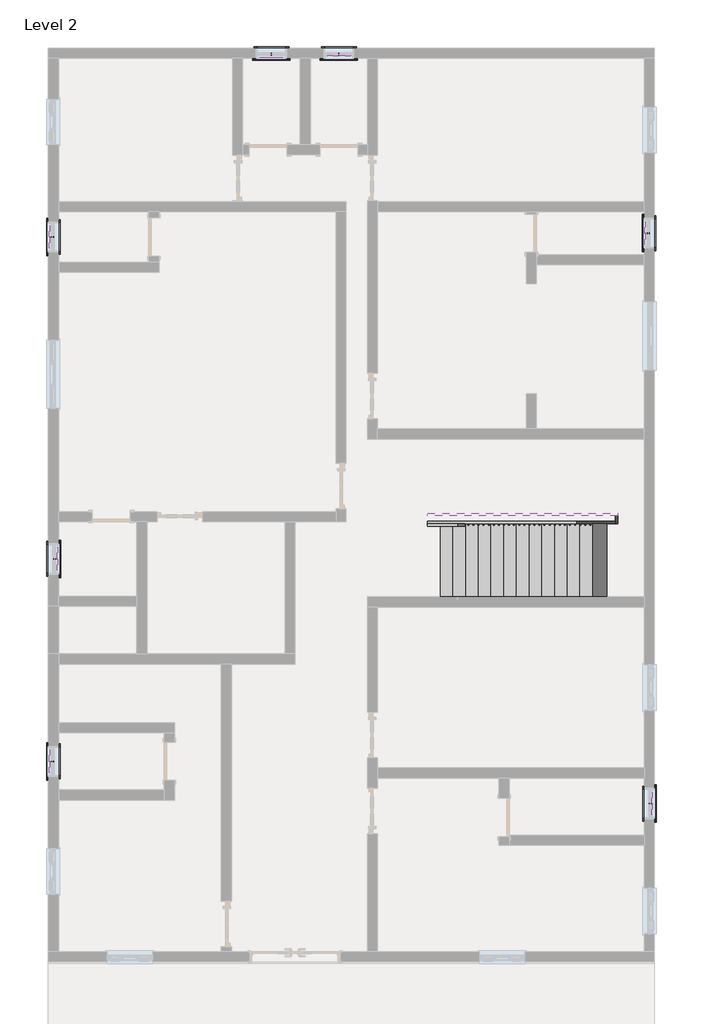
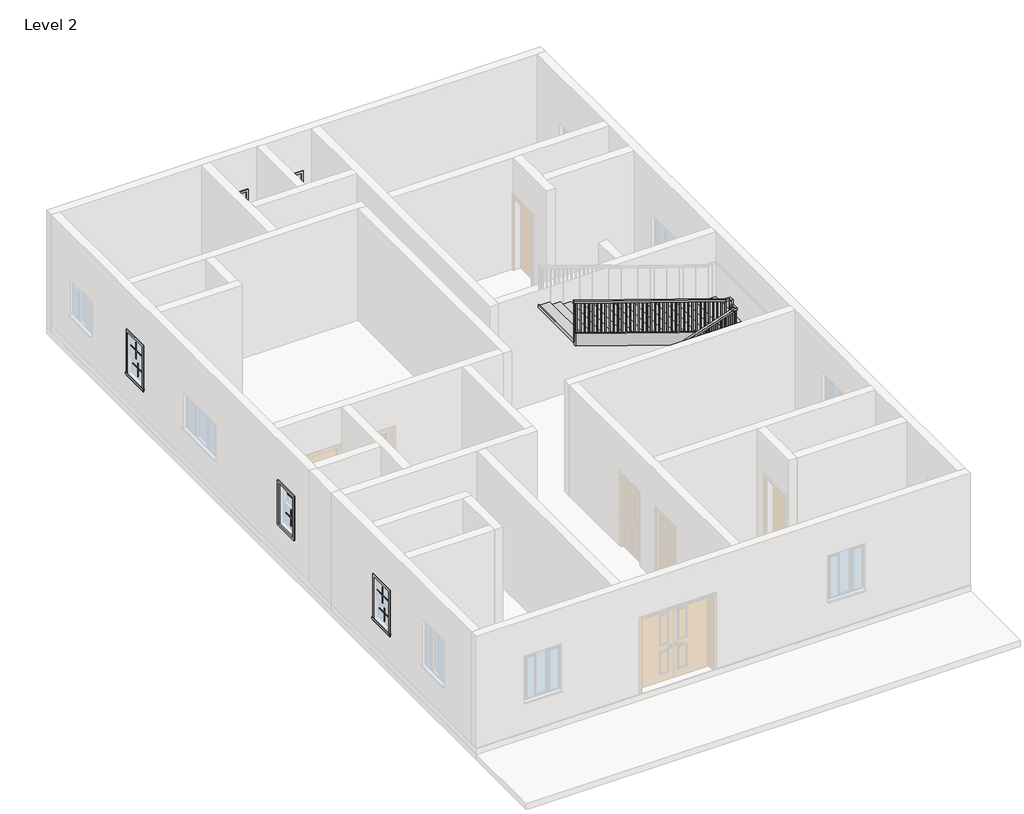
# One storey, part 3 of 3: 28 proxies, 6 members, 1 railing, 1 stair flight.
"""IFC4 building model written with IfcOpenShell, lengths in millimetres."""

from ifc_helpers import new_model, si_unit, frame, origin, place, context, project, spatial, polyline, outline, extrude, faceted_brep, transform, mapped, element, save
from components import muntin_pattern_2x2_muntin_pattern_2x2_eba6c5fb, trim_window_exterior_flat_with_sill_278e6a94, trim_window_interior_flat_picture_frame_e9fd5f45, stair_flight_4f1afc7f

model = new_model("IFC4")

# Units and contexts
model_context = context("Model", 3, world=origin())
ifc_project = project(units=[si_unit("LENGTHUNIT", "METRE", prefix="MILLI")], contexts=[model_context])

# Site, building, storey
site = spatial("IfcSite", under=ifc_project)
building = spatial("IfcBuilding", under=site)
storey = spatial("IfcBuildingStorey", under=building, Name="Level 2", Elevation=3048.0)

# Proxies
placement = place(None, origin())
muntin_pattern_2x2_muntin_pattern_2x2_shape = muntin_pattern_2x2_muntin_pattern_2x2_eba6c5fb(model_context)
element("IfcBuildingElementProxy", 1, Name="Muntin Pattern_2x2 : Muntin Pattern_2x2", ObjectType="Muntin Pattern_2x2 : Muntin Pattern_2x2", at=placement, inside=storey, context=model_context, shape_type="MappedRepresentation", body=[
    mapped(muntin_pattern_2x2_muntin_pattern_2x2_shape, transform((-6096.8589448, 5183.1303322, 4518.025), x_axis=(0.0, 1.0, 0.0), y_axis=(-1.0, 0.0, 0.0), z_axis=(0.0, 0.0, 1.0))),
])
element("IfcBuildingElementProxy", 2, Name="Muntin Pattern_2x2 : Muntin Pattern_2x2", ObjectType="Muntin Pattern_2x2 : Muntin Pattern_2x2", at=placement, inside=storey, context=model_context, shape_type="MappedRepresentation", body=[
    mapped(muntin_pattern_2x2_muntin_pattern_2x2_shape, transform((-6052.4089448, 5183.1303322, 4038.6), x_axis=(0.0, 1.0, 0.0), y_axis=(-1.0, 0.0, 0.0), z_axis=(0.0, 0.0, 1.0))),
])
element("IfcBuildingElementProxy", 3, Name="Muntin Pattern_2x2 : Muntin Pattern_2x2", ObjectType="Muntin Pattern_2x2 : Muntin Pattern_2x2", at=placement, inside=storey, context=model_context, shape_type="MappedRepresentation", body=[
    mapped(muntin_pattern_2x2_muntin_pattern_2x2_shape, transform((-1673.5309118, 8787.5224079, 4518.025), x_axis=(-1.0, 0.0, 0.0), y_axis=(0.0, -1.0, 0.0), z_axis=(0.0, 0.0, 1.0))),
])
element("IfcBuildingElementProxy", 4, Name="Muntin Pattern_2x2 : Muntin Pattern_2x2", ObjectType="Muntin Pattern_2x2 : Muntin Pattern_2x2", at=placement, inside=storey, context=model_context, shape_type="MappedRepresentation", body=[
    mapped(muntin_pattern_2x2_muntin_pattern_2x2_shape, transform((-1673.5309118, 8831.9724079, 4038.6), x_axis=(-1.0, 0.0, 0.0), y_axis=(0.0, -1.0, 0.0), z_axis=(0.0, 0.0, 1.0))),
])
element("IfcBuildingElementProxy", 5, Name="Muntin Pattern_2x2 : Muntin Pattern_2x2", ObjectType="Muntin Pattern_2x2 : Muntin Pattern_2x2", at=placement, inside=storey, context=model_context, shape_type="MappedRepresentation", body=[
    mapped(muntin_pattern_2x2_muntin_pattern_2x2_shape, transform((-324.5451949, 8787.5224079, 4518.025), x_axis=(-1.0, 0.0, 0.0), y_axis=(0.0, -1.0, 0.0), z_axis=(0.0, 0.0, 1.0))),
])
element("IfcBuildingElementProxy", 6, Name="Muntin Pattern_2x2 : Muntin Pattern_2x2", ObjectType="Muntin Pattern_2x2 : Muntin Pattern_2x2", at=placement, inside=storey, context=model_context, shape_type="MappedRepresentation", body=[
    mapped(muntin_pattern_2x2_muntin_pattern_2x2_shape, transform((-324.5451949, 8831.9724079, 4038.6), x_axis=(-1.0, 0.0, 0.0), y_axis=(0.0, -1.0, 0.0), z_axis=(0.0, 0.0, 1.0))),
])
element("IfcBuildingElementProxy", 7, Name="Muntin Pattern_2x2 : Muntin Pattern_2x2", ObjectType="Muntin Pattern_2x2 : Muntin Pattern_2x2", at=placement, inside=storey, context=model_context, shape_type="MappedRepresentation", body=[
    mapped(muntin_pattern_2x2_muntin_pattern_2x2_shape, transform((5813.4689795, 5259.3303322, 4518.025), x_axis=(0.0, 1.0, 0.0), y_axis=(-1.0, 0.0, 0.0), z_axis=(0.0, 0.0, 1.0))),
])
element("IfcBuildingElementProxy", 8, Name="Muntin Pattern_2x2 : Muntin Pattern_2x2", ObjectType="Muntin Pattern_2x2 : Muntin Pattern_2x2", at=placement, inside=storey, context=model_context, shape_type="MappedRepresentation", body=[
    mapped(muntin_pattern_2x2_muntin_pattern_2x2_shape, transform((5857.9189795, 5259.3303322, 4038.6), x_axis=(0.0, 1.0, 0.0), y_axis=(-1.0, 0.0, 0.0), z_axis=(0.0, 0.0, 1.0))),
])
element("IfcBuildingElementProxy", 9, Name="Muntin Pattern_2x2 : Muntin Pattern_2x2", ObjectType="Muntin Pattern_2x2 : Muntin Pattern_2x2", at=placement, inside=storey, context=model_context, shape_type="MappedRepresentation", body=[
    mapped(muntin_pattern_2x2_muntin_pattern_2x2_shape, transform((5946.8189795, -6133.2488489, 4518.025), x_axis=(0.0, -1.0, 0.0), y_axis=(1.0, 0.0, 0.0), z_axis=(0.0, 0.0, 1.0))),
])
element("IfcBuildingElementProxy", 10, Name="Muntin Pattern_2x2 : Muntin Pattern_2x2", ObjectType="Muntin Pattern_2x2 : Muntin Pattern_2x2", at=placement, inside=storey, context=model_context, shape_type="MappedRepresentation", body=[
    mapped(muntin_pattern_2x2_muntin_pattern_2x2_shape, transform((5902.3689795, -6133.2488489, 4038.6), x_axis=(0.0, -1.0, 0.0), y_axis=(1.0, 0.0, 0.0), z_axis=(0.0, 0.0, 1.0))),
])
element("IfcBuildingElementProxy", 11, Name="Muntin Pattern_2x2 : Muntin Pattern_2x2", ObjectType="Muntin Pattern_2x2 : Muntin Pattern_2x2", at=placement, inside=storey, context=model_context, shape_type="MappedRepresentation", body=[
    mapped(muntin_pattern_2x2_muntin_pattern_2x2_shape, transform((-6096.8589448, -5291.0659014, 4518.025), x_axis=(0.0, 1.0, 0.0), y_axis=(-1.0, 0.0, 0.0), z_axis=(0.0, 0.0, 1.0))),
])
element("IfcBuildingElementProxy", 12, Name="Muntin Pattern_2x2 : Muntin Pattern_2x2", ObjectType="Muntin Pattern_2x2 : Muntin Pattern_2x2", at=placement, inside=storey, context=model_context, shape_type="MappedRepresentation", body=[
    mapped(muntin_pattern_2x2_muntin_pattern_2x2_shape, transform((-6052.4089448, -5291.0659014, 4038.6), x_axis=(0.0, 1.0, 0.0), y_axis=(-1.0, 0.0, 0.0), z_axis=(0.0, 0.0, 1.0))),
])
element("IfcBuildingElementProxy", 13, Name="Muntin Pattern_2x2 : Muntin Pattern_2x2", ObjectType="Muntin Pattern_2x2 : Muntin Pattern_2x2", at=placement, inside=storey, context=model_context, shape_type="MappedRepresentation", body=[
    mapped(muntin_pattern_2x2_muntin_pattern_2x2_shape, transform((-5963.5089448, -1246.1159014, 4518.025), x_axis=(0.0, -1.0, 0.0), y_axis=(1.0, 0.0, 0.0), z_axis=(0.0, 0.0, 1.0))),
])
element("IfcBuildingElementProxy", 14, Name="Muntin Pattern_2x2 : Muntin Pattern_2x2", ObjectType="Muntin Pattern_2x2 : Muntin Pattern_2x2", at=placement, inside=storey, context=model_context, shape_type="MappedRepresentation", body=[
    mapped(muntin_pattern_2x2_muntin_pattern_2x2_shape, transform((-6007.9589448, -1246.1159014, 4038.6), x_axis=(0.0, -1.0, 0.0), y_axis=(1.0, 0.0, 0.0), z_axis=(0.0, 0.0, 1.0))),
])
trim_window_exterior_flat_with_sill_shape = trim_window_exterior_flat_with_sill_278e6a94(model_context)
element("IfcBuildingElementProxy", 15, Name="Trim-Window-Exterior-Flat : with Sill", ObjectType="Trim-Window-Exterior-Flat : with Sill", at=placement, inside=storey, context=model_context, shape_type="MappedRepresentation", body=[
    mapped(trim_window_exterior_flat_with_sill_shape, transform((-6131.7839448, 5183.1303322, 5029.2), x_axis=(0.0, -1.0, 0.0), y_axis=(0.0, 0.0, 1.0), z_axis=(-1.0, 0.0, 0.0))),
])
element("IfcBuildingElementProxy", 16, Name="Trim-Window-Exterior-Flat : with Sill", ObjectType="Trim-Window-Exterior-Flat : with Sill", at=placement, inside=storey, context=model_context, shape_type="MappedRepresentation", body=[
    mapped(trim_window_exterior_flat_with_sill_shape, transform((-1673.5309118, 8752.5974079, 5029.2), x_axis=(1.0, 0.0, 0.0), y_axis=(0.0, 0.0, 1.0), z_axis=(0.0, -1.0, 0.0))),
])
element("IfcBuildingElementProxy", 17, Name="Trim-Window-Exterior-Flat : with Sill", ObjectType="Trim-Window-Exterior-Flat : with Sill", at=placement, inside=storey, context=model_context, shape_type="MappedRepresentation", body=[
    mapped(trim_window_exterior_flat_with_sill_shape, transform((-324.5451949, 8752.5974079, 5029.2), x_axis=(1.0, 0.0, 0.0), y_axis=(0.0, 0.0, 1.0), z_axis=(0.0, -1.0, 0.0))),
])
element("IfcBuildingElementProxy", 18, Name="Trim-Window-Exterior-Flat : with Sill", ObjectType="Trim-Window-Exterior-Flat : with Sill", at=placement, inside=storey, context=model_context, shape_type="MappedRepresentation", body=[
    mapped(trim_window_exterior_flat_with_sill_shape, transform((5778.5439795, 5259.3303322, 5029.2), x_axis=(0.0, -1.0, 0.0), y_axis=(0.0, 0.0, 1.0), z_axis=(-1.0, 0.0, 0.0))),
])
element("IfcBuildingElementProxy", 19, Name="Trim-Window-Exterior-Flat : with Sill", ObjectType="Trim-Window-Exterior-Flat : with Sill", at=placement, inside=storey, context=model_context, shape_type="MappedRepresentation", body=[
    mapped(trim_window_exterior_flat_with_sill_shape, transform((5981.7439795, -6133.2488489, 5029.2), x_axis=(0.0, 1.0, 0.0), y_axis=(0.0, 0.0, 1.0), z_axis=(1.0, 0.0, 0.0))),
])
element("IfcBuildingElementProxy", 20, Name="Trim-Window-Exterior-Flat : with Sill", ObjectType="Trim-Window-Exterior-Flat : with Sill", at=placement, inside=storey, context=model_context, shape_type="MappedRepresentation", body=[
    mapped(trim_window_exterior_flat_with_sill_shape, transform((-6131.7839448, -5291.0659014, 5029.2), x_axis=(0.0, -1.0, 0.0), y_axis=(0.0, 0.0, 1.0), z_axis=(-1.0, 0.0, 0.0))),
])
element("IfcBuildingElementProxy", 21, Name="Trim-Window-Exterior-Flat : with Sill", ObjectType="Trim-Window-Exterior-Flat : with Sill", at=placement, inside=storey, context=model_context, shape_type="MappedRepresentation", body=[
    mapped(trim_window_exterior_flat_with_sill_shape, transform((-5928.5839448, -1246.1159014, 5029.2), x_axis=(0.0, 1.0, 0.0), y_axis=(0.0, 0.0, 1.0), z_axis=(1.0, 0.0, 0.0))),
])
trim_window_interior_flat_picture_frame_shape = trim_window_interior_flat_picture_frame_e9fd5f45(model_context)
element("IfcBuildingElementProxy", 22, Name="Trim-Window-Interior-Flat : Picture Frame", ObjectType="Trim-Window-Interior-Flat : Picture Frame", at=placement, inside=storey, context=model_context, shape_type="MappedRepresentation", body=[
    mapped(trim_window_interior_flat_picture_frame_shape, transform((-5928.5839448, 5183.1303322, 5029.2), x_axis=(0.0, 1.0, 0.0), y_axis=(0.0, 0.0, 1.0), z_axis=(1.0, 0.0, 0.0))),
])
element("IfcBuildingElementProxy", 23, Name="Trim-Window-Interior-Flat : Picture Frame", ObjectType="Trim-Window-Interior-Flat : Picture Frame", at=placement, inside=storey, context=model_context, shape_type="MappedRepresentation", body=[
    mapped(trim_window_interior_flat_picture_frame_shape, transform((-1673.5309118, 8955.7974079, 5029.2), x_axis=(-1.0, 0.0, 0.0), y_axis=(0.0, 0.0, 1.0), z_axis=(0.0, 1.0, 0.0))),
])
element("IfcBuildingElementProxy", 24, Name="Trim-Window-Interior-Flat : Picture Frame", ObjectType="Trim-Window-Interior-Flat : Picture Frame", at=placement, inside=storey, context=model_context, shape_type="MappedRepresentation", body=[
    mapped(trim_window_interior_flat_picture_frame_shape, transform((-324.5451949, 8955.7974079, 5029.2), x_axis=(-1.0, 0.0, 0.0), y_axis=(0.0, 0.0, 1.0), z_axis=(0.0, 1.0, 0.0))),
])
element("IfcBuildingElementProxy", 25, Name="Trim-Window-Interior-Flat : Picture Frame", ObjectType="Trim-Window-Interior-Flat : Picture Frame", at=placement, inside=storey, context=model_context, shape_type="MappedRepresentation", body=[
    mapped(trim_window_interior_flat_picture_frame_shape, transform((5981.7439795, 5259.3303322, 5029.2), x_axis=(0.0, 1.0, 0.0), y_axis=(0.0, 0.0, 1.0), z_axis=(1.0, 0.0, 0.0))),
])
element("IfcBuildingElementProxy", 26, Name="Trim-Window-Interior-Flat : Picture Frame", ObjectType="Trim-Window-Interior-Flat : Picture Frame", at=placement, inside=storey, context=model_context, shape_type="MappedRepresentation", body=[
    mapped(trim_window_interior_flat_picture_frame_shape, transform((5778.5439795, -6133.2488489, 5029.2), x_axis=(0.0, -1.0, 0.0), y_axis=(0.0, 0.0, 1.0), z_axis=(-1.0, 0.0, 0.0))),
])
element("IfcBuildingElementProxy", 27, Name="Trim-Window-Interior-Flat : Picture Frame", ObjectType="Trim-Window-Interior-Flat : Picture Frame", at=placement, inside=storey, context=model_context, shape_type="MappedRepresentation", body=[
    mapped(trim_window_interior_flat_picture_frame_shape, transform((-5928.5839448, -5291.0659014, 5029.2), x_axis=(0.0, 1.0, 0.0), y_axis=(0.0, 0.0, 1.0), z_axis=(1.0, 0.0, 0.0))),
])
element("IfcBuildingElementProxy", 28, Name="Trim-Window-Interior-Flat : Picture Frame", ObjectType="Trim-Window-Interior-Flat : Picture Frame", at=placement, inside=storey, context=model_context, shape_type="MappedRepresentation", body=[
    mapped(trim_window_interior_flat_picture_frame_shape, transform((-6131.7839448, -1246.1159014, 5029.2), x_axis=(0.0, -1.0, 0.0), y_axis=(0.0, 0.0, 1.0), z_axis=(-1.0, 0.0, 0.0))),
])

# Members
element("IfcMember", 29, ObjectType="Stringer - 2\" Width", at=placement, inside=storey, context=model_context, shape_type="SweptSolid", body=[
    extrude(outline(polyline([(3241.7751932, 1449.3932247), (3048.0, 1449.3932247), (3048.0, 1827.5890963), (4188.094539, 5195.8669505), (4495.8, 5195.8669505), (4495.8, 5154.2649181), (3241.7751932, 1449.3932247)])), frame((0.0, -541.2659014, 0.0), z_axis=(0.0, 1.0, 0.0), x_axis=(0.0, 0.0, 1.0)), (0.0, 0.0, 1.0), 50.8),
])
element("IfcMember", 30, ObjectType="Stringer - 2\" Width", at=placement, inside=storey, context=model_context, shape_type="SweptSolid", body=[
    extrude(outline(polyline([(5246.6669505, -541.2659014), (5195.8669505, -541.2659014), (5195.8669505, -388.7910016), (5246.6669505, -388.7910016), (5246.6669505, -541.2659014)])), frame((0.0, 0.0, 4191.0), z_axis=(0.0, 0.0, 1.0), x_axis=(1.0, 0.0, 0.0)), (0.0, 0.0, 1.0), 304.8),
])
element("IfcMember", 31, ObjectType="Stringer - 2\" Width", at=placement, inside=storey, context=model_context, shape_type="SweptSolid", body=[
    extrude(outline(polyline([(4291.0143208, 5246.6669505), (4612.8012358, 5246.6669505), (5898.1022784, 1449.3932247), (5576.3153634, 1449.3932247), (4291.0143208, 5246.6669505)])), frame((0.0, -388.7910016, 0.0), z_axis=(0.0, 1.0, 0.0), x_axis=(0.0, 0.0, 1.0)), (0.0, 0.0, 1.0), 50.8),
])
element("IfcMember", 32, ObjectType="Stringer - 2\" Width", at=placement, inside=storey, context=model_context, shape_type="SweptSolid", body=[
    extrude(outline(polyline([(3241.7751932, 1449.3932247), (3048.0, 1449.3932247), (3048.0, 1827.5890963), (4400.1142723, 5822.2548051), (4495.8, 5822.2548051), (4495.8, 5154.2649181), (3241.7751932, 1449.3932247)])), frame((0.0, -2116.0659014, 0.0), z_axis=(0.0, 1.0, 0.0), x_axis=(0.0, 0.0, 1.0)), (0.0, 0.0, 1.0), 50.8),
])
element("IfcMember", 33, ObjectType="Stringer - 2\" Width", at=placement, inside=storey, context=model_context, shape_type="SweptSolid", body=[
    extrude(outline(polyline([(5873.0548051, -2116.0659014), (5822.2548051, -2116.0659014), (5822.2548051, 1185.9340986), (5873.0548051, 1185.9340986), (5873.0548051, -2116.0659014)])), frame((0.0, 0.0, 4191.0), z_axis=(0.0, 0.0, 1.0), x_axis=(1.0, 0.0, 0.0)), (0.0, 0.0, 1.0), 304.8),
])
element("IfcMember", 34, ObjectType="Stringer - 2\" Width", at=placement, inside=storey, context=model_context, shape_type="SweptSolid", body=[
    extrude(outline(polyline([(4191.0, 5873.0548051), (4400.7815025, 5873.0548051), (5898.1022784, 1449.3932247), (5576.3153634, 1449.3932247), (4191.0, 5542.1477288), (4191.0, 5873.0548051)])), frame((0.0, 1185.9340986, 0.0), z_axis=(0.0, 1.0, 0.0), x_axis=(0.0, 0.0, 1.0)), (0.0, 0.0, 1.0), 50.8),
])

# Railing
element("IfcRailing", 35, ObjectType="Handrail - Rectangular", at=placement, inside=storey, context=model_context, shape_type="SolidModel", body=[
    faceted_brep([(1449.3932247, -541.2659014, 4048.125), (1449.3932247, -541.2659014, 3994.4913852), (1449.3932247, -592.0659014, 3994.4913852), (1449.3932247, -592.0659014, 4048.125), (5170.4669505, -541.2659014, 5308.1963098), (5221.2669505, -541.2659014, 5271.7651551), (5221.2669505, -592.0659014, 5271.7651551), (5170.4669505, -592.0659014, 5308.1963098), (5170.4669505, -541.2659014, 5334.0), (5221.2669505, -541.2659014, 5283.2), (5221.2669505, -592.0659014, 5283.2), (5170.4669505, -592.0659014, 5334.0), (5246.6669505, -541.2659014, 5334.0), (5246.6669505, -541.2659014, 5283.2), (5297.4669505, -592.0659014, 5283.2), (5297.4669505, -592.0659014, 5334.0), (5246.6669505, -465.0659014, 5334.0), (5246.6669505, -465.0659014, 5283.2), (5297.4669505, -465.0659014, 5283.2), (5297.4669505, -465.0659014, 5334.0), (5246.6669505, -414.1910016, 5334.0), (5246.6669505, -363.3910016, 5283.2), (5297.4669505, -363.3910016, 5283.2), (5297.4669505, -414.1910016, 5334.0), (5246.6669505, -414.1910016, 5445.5286902), (5246.6669505, -363.3910016, 5394.7286902), (5297.4669505, -363.3910016, 5394.7286902), (5297.4669505, -414.1910016, 5445.5286902), (5246.6669505, -337.9910016, 5445.5286902), (5246.6669505, -337.9910016, 5394.7286902), (5297.4669505, -287.1910016, 5394.7286902), (5297.4669505, -287.1910016, 5445.5286902), (5170.4669505, -337.9910016, 5445.5286902), (5162.099099, -337.9910016, 5394.7286902), (5162.099099, -287.1910016, 5394.7286902), (5170.4669505, -287.1910016, 5445.5286902), (1449.3932247, -337.9910016, 6705.6), (1449.3932247, -287.1910016, 6705.6), (1449.3932247, -287.1910016, 6651.9663852), (1449.3932247, -337.9910016, 6651.9663852)], [[[0, 1, 2, 3]], [[1, 0, 4, 5]], [[2, 1, 5, 6]], [[3, 2, 6, 7]], [[0, 3, 7, 4]], [[5, 4, 8, 9]], [[6, 5, 9, 10]], [[7, 6, 10, 11]], [[4, 7, 11, 8]], [[9, 8, 12, 13]], [[10, 9, 13, 14]], [[11, 10, 14, 15]], [[8, 11, 15, 12]], [[13, 12, 16, 17]], [[14, 13, 17, 18]], [[15, 14, 18, 19]], [[12, 15, 19, 16]], [[17, 16, 20, 21]], [[18, 17, 21, 22]], [[19, 18, 22, 23]], [[16, 19, 23, 20]], [[21, 20, 24, 25]], [[22, 21, 25, 26]], [[23, 22, 26, 27]], [[20, 23, 27, 24]], [[25, 24, 28, 29]], [[26, 25, 29, 30]], [[27, 26, 30, 31]], [[24, 27, 31, 28]], [[29, 28, 32, 33]], [[30, 29, 33, 34]], [[31, 30, 34, 35]], [[28, 31, 35, 32]], [[36, 37, 38, 39]], [[33, 32, 36, 39]], [[34, 33, 39, 38]], [[35, 34, 38, 37]], [[32, 35, 37, 36]]]),
    extrude(outline(polyline([(6633.6976686, 1503.3419505), (5705.475, 1503.3419505), (5705.475, 1522.3919505), (6627.246746, 1522.3919505), (6633.6976686, 1503.3419505)])), frame((0.0, -322.1160016, 0.0), z_axis=(0.0, 1.0, 0.0), x_axis=(0.0, 0.0, 1.0)), (0.0, 0.0, 1.0), 19.05),
    extrude(outline(polyline([(6599.2927482, 1604.9419505), (5705.475, 1604.9419505), (5705.475, 1623.9919505), (6592.8418257, 1623.9919505), (6599.2927482, 1604.9419505)])), frame((0.0, -322.1160016, 0.0), z_axis=(0.0, 1.0, 0.0), x_axis=(0.0, 0.0, 1.0)), (0.0, 0.0, 1.0), 19.05),
    extrude(outline(polyline([(6564.8878279, 1706.5419505), (5619.75, 1706.5419505), (5619.75, 1725.5919505), (6558.4369054, 1725.5919505), (6564.8878279, 1706.5419505)])), frame((0.0, -322.1160016, 0.0), z_axis=(0.0, 1.0, 0.0), x_axis=(0.0, 0.0, 1.0)), (0.0, 0.0, 1.0), 19.05),
    extrude(outline(polyline([(6530.4829076, 1808.1419505), (5619.75, 1808.1419505), (5619.75, 1827.1919505), (6524.031985, 1827.1919505), (6530.4829076, 1808.1419505)])), frame((0.0, -322.1160016, 0.0), z_axis=(0.0, 1.0, 0.0), x_axis=(0.0, 0.0, 1.0)), (0.0, 0.0, 1.0), 19.05),
    extrude(outline(polyline([(6496.0779873, 1909.7419505), (5619.75, 1909.7419505), (5619.75, 1928.7919505), (6489.6270647, 1928.7919505), (6496.0779873, 1909.7419505)])), frame((0.0, -322.1160016, 0.0), z_axis=(0.0, 1.0, 0.0), x_axis=(0.0, 0.0, 1.0)), (0.0, 0.0, 1.0), 19.05),
    extrude(outline(polyline([(6461.6730669, 2011.3419505), (5534.025, 2011.3419505), (5534.025, 2030.3919505), (6455.2221444, 2030.3919505), (6461.6730669, 2011.3419505)])), frame((0.0, -322.1160016, 0.0), z_axis=(0.0, 1.0, 0.0), x_axis=(0.0, 0.0, 1.0)), (0.0, 0.0, 1.0), 19.05),
    extrude(outline(polyline([(6427.2681466, 2112.9419505), (5534.025, 2112.9419505), (5534.025, 2131.9919505), (6420.817224, 2131.9919505), (6427.2681466, 2112.9419505)])), frame((0.0, -322.1160016, 0.0), z_axis=(0.0, 1.0, 0.0), x_axis=(0.0, 0.0, 1.0)), (0.0, 0.0, 1.0), 19.05),
    extrude(outline(polyline([(6392.8632263, 2214.5419505), (5448.3, 2214.5419505), (5448.3, 2233.5919505), (6386.4123037, 2233.5919505), (6392.8632263, 2214.5419505)])), frame((0.0, -322.1160016, 0.0), z_axis=(0.0, 1.0, 0.0), x_axis=(0.0, 0.0, 1.0)), (0.0, 0.0, 1.0), 19.05),
    extrude(outline(polyline([(6358.4583059, 2316.1419505), (5448.3, 2316.1419505), (5448.3, 2335.1919505), (6352.0073834, 2335.1919505), (6358.4583059, 2316.1419505)])), frame((0.0, -322.1160016, 0.0), z_axis=(0.0, 1.0, 0.0), x_axis=(0.0, 0.0, 1.0)), (0.0, 0.0, 1.0), 19.05),
    extrude(outline(polyline([(6324.0533856, 2417.7419505), (5448.3, 2417.7419505), (5448.3, 2436.7919505), (6317.6024631, 2436.7919505), (6324.0533856, 2417.7419505)])), frame((0.0, -322.1160016, 0.0), z_axis=(0.0, 1.0, 0.0), x_axis=(0.0, 0.0, 1.0)), (0.0, 0.0, 1.0), 19.05),
    extrude(outline(polyline([(6289.6484653, 2519.3419505), (5362.575, 2519.3419505), (5362.575, 2538.3919505), (6283.1975427, 2538.3919505), (6289.6484653, 2519.3419505)])), frame((0.0, -322.1160016, 0.0), z_axis=(0.0, 1.0, 0.0), x_axis=(0.0, 0.0, 1.0)), (0.0, 0.0, 1.0), 19.05),
    extrude(outline(polyline([(6255.243545, 2620.9419505), (5362.575, 2620.9419505), (5362.575, 2639.9919505), (6248.7926224, 2639.9919505), (6255.243545, 2620.9419505)])), frame((0.0, -322.1160016, 0.0), z_axis=(0.0, 1.0, 0.0), x_axis=(0.0, 0.0, 1.0)), (0.0, 0.0, 1.0), 19.05),
    extrude(outline(polyline([(6220.8386246, 2722.5419505), (5276.85, 2722.5419505), (5276.85, 2741.5919505), (6214.3877021, 2741.5919505), (6220.8386246, 2722.5419505)])), frame((0.0, -322.1160016, 0.0), z_axis=(0.0, 1.0, 0.0), x_axis=(0.0, 0.0, 1.0)), (0.0, 0.0, 1.0), 19.05),
    extrude(outline(polyline([(6186.4337043, 2824.1419505), (5276.85, 2824.1419505), (5276.85, 2843.1919505), (6179.9827817, 2843.1919505), (6186.4337043, 2824.1419505)])), frame((0.0, -322.1160016, 0.0), z_axis=(0.0, 1.0, 0.0), x_axis=(0.0, 0.0, 1.0)), (0.0, 0.0, 1.0), 19.05),
    extrude(outline(polyline([(6152.028784, 2925.7419505), (5276.85, 2925.7419505), (5276.85, 2944.7919505), (6145.5778614, 2944.7919505), (6152.028784, 2925.7419505)])), frame((0.0, -322.1160016, 0.0), z_axis=(0.0, 1.0, 0.0), x_axis=(0.0, 0.0, 1.0)), (0.0, 0.0, 1.0), 19.05),
    extrude(outline(polyline([(6117.6238636, 3027.3419505), (5191.125, 3027.3419505), (5191.125, 3046.3919505), (6111.1729411, 3046.3919505), (6117.6238636, 3027.3419505)])), frame((0.0, -322.1160016, 0.0), z_axis=(0.0, 1.0, 0.0), x_axis=(0.0, 0.0, 1.0)), (0.0, 0.0, 1.0), 19.05),
    extrude(outline(polyline([(6083.2189433, 3128.9419505), (5191.125, 3128.9419505), (5191.125, 3147.9919505), (6076.7680208, 3147.9919505), (6083.2189433, 3128.9419505)])), frame((0.0, -322.1160016, 0.0), z_axis=(0.0, 1.0, 0.0), x_axis=(0.0, 0.0, 1.0)), (0.0, 0.0, 1.0), 19.05),
    extrude(outline(polyline([(6048.814023, 3230.5419505), (5105.4, 3230.5419505), (5105.4, 3249.5919505), (6042.3631004, 3249.5919505), (6048.814023, 3230.5419505)])), frame((0.0, -322.1160016, 0.0), z_axis=(0.0, 1.0, 0.0), x_axis=(0.0, 0.0, 1.0)), (0.0, 0.0, 1.0), 19.05),
    extrude(outline(polyline([(6014.4091027, 3332.1419505), (5105.4, 3332.1419505), (5105.4, 3351.1919505), (6007.9581801, 3351.1919505), (6014.4091027, 3332.1419505)])), frame((0.0, -322.1160016, 0.0), z_axis=(0.0, 1.0, 0.0), x_axis=(0.0, 0.0, 1.0)), (0.0, 0.0, 1.0), 19.05),
    extrude(outline(polyline([(5980.0041823, 3433.7419505), (5105.4, 3433.7419505), (5105.4, 3452.7919505), (5973.5532598, 3452.7919505), (5980.0041823, 3433.7419505)])), frame((0.0, -322.1160016, 0.0), z_axis=(0.0, 1.0, 0.0), x_axis=(0.0, 0.0, 1.0)), (0.0, 0.0, 1.0), 19.05),
    extrude(outline(polyline([(5945.599262, 3535.3419505), (5019.675, 3535.3419505), (5019.675, 3554.3919505), (5939.1483394, 3554.3919505), (5945.599262, 3535.3419505)])), frame((0.0, -322.1160016, 0.0), z_axis=(0.0, 1.0, 0.0), x_axis=(0.0, 0.0, 1.0)), (0.0, 0.0, 1.0), 19.05),
    extrude(outline(polyline([(5911.1943417, 3636.9419505), (5019.675, 3636.9419505), (5019.675, 3655.9919505), (5904.7434191, 3655.9919505), (5911.1943417, 3636.9419505)])), frame((0.0, -322.1160016, 0.0), z_axis=(0.0, 1.0, 0.0), x_axis=(0.0, 0.0, 1.0)), (0.0, 0.0, 1.0), 19.05),
    extrude(outline(polyline([(5876.7894213, 3738.5419505), (4933.95, 3738.5419505), (4933.95, 3757.5919505), (5870.3384988, 3757.5919505), (5876.7894213, 3738.5419505)])), frame((0.0, -322.1160016, 0.0), z_axis=(0.0, 1.0, 0.0), x_axis=(0.0, 0.0, 1.0)), (0.0, 0.0, 1.0), 19.05),
    extrude(outline(polyline([(5842.384501, 3840.1419505), (4933.95, 3840.1419505), (4933.95, 3859.1919505), (5835.9335784, 3859.1919505), (5842.384501, 3840.1419505)])), frame((0.0, -322.1160016, 0.0), z_axis=(0.0, 1.0, 0.0), x_axis=(0.0, 0.0, 1.0)), (0.0, 0.0, 1.0), 19.05),
    extrude(outline(polyline([(5807.9795807, 3941.7419505), (4933.95, 3941.7419505), (4933.95, 3960.7919505), (5801.5286581, 3960.7919505), (5807.9795807, 3941.7419505)])), frame((0.0, -322.1160016, 0.0), z_axis=(0.0, 1.0, 0.0), x_axis=(0.0, 0.0, 1.0)), (0.0, 0.0, 1.0), 19.05),
    extrude(outline(polyline([(5773.5746604, 4043.3419505), (4848.225, 4043.3419505), (4848.225, 4062.3919505), (5767.1237378, 4062.3919505), (5773.5746604, 4043.3419505)])), frame((0.0, -322.1160016, 0.0), z_axis=(0.0, 1.0, 0.0), x_axis=(0.0, 0.0, 1.0)), (0.0, 0.0, 1.0), 19.05),
    extrude(outline(polyline([(5739.16974, 4144.9419505), (4848.225, 4144.9419505), (4848.225, 4163.9919505), (5732.7188175, 4163.9919505), (5739.16974, 4144.9419505)])), frame((0.0, -322.1160016, 0.0), z_axis=(0.0, 1.0, 0.0), x_axis=(0.0, 0.0, 1.0)), (0.0, 0.0, 1.0), 19.05),
    extrude(outline(polyline([(5704.7648197, 4246.5419505), (4762.5, 4246.5419505), (4762.5, 4265.5919505), (5698.3138971, 4265.5919505), (5704.7648197, 4246.5419505)])), frame((0.0, -322.1160016, 0.0), z_axis=(0.0, 1.0, 0.0), x_axis=(0.0, 0.0, 1.0)), (0.0, 0.0, 1.0), 19.05),
    extrude(outline(polyline([(5670.3598994, 4348.1419505), (4762.5, 4348.1419505), (4762.5, 4367.1919505), (5663.9089768, 4367.1919505), (5670.3598994, 4348.1419505)])), frame((0.0, -322.1160016, 0.0), z_axis=(0.0, 1.0, 0.0), x_axis=(0.0, 0.0, 1.0)), (0.0, 0.0, 1.0), 19.05),
    extrude(outline(polyline([(5635.954979, 4449.7419505), (4762.5, 4449.7419505), (4762.5, 4468.7919505), (5629.5040565, 4468.7919505), (5635.954979, 4449.7419505)])), frame((0.0, -322.1160016, 0.0), z_axis=(0.0, 1.0, 0.0), x_axis=(0.0, 0.0, 1.0)), (0.0, 0.0, 1.0), 19.05),
    extrude(outline(polyline([(5601.5500587, 4551.3419505), (4676.775, 4551.3419505), (4676.775, 4570.3919505), (5595.0991361, 4570.3919505), (5601.5500587, 4551.3419505)])), frame((0.0, -322.1160016, 0.0), z_axis=(0.0, 1.0, 0.0), x_axis=(0.0, 0.0, 1.0)), (0.0, 0.0, 1.0), 19.05),
    extrude(outline(polyline([(5567.1451384, 4652.9419505), (4676.775, 4652.9419505), (4676.775, 4671.9919505), (5560.6942158, 4671.9919505), (5567.1451384, 4652.9419505)])), frame((0.0, -322.1160016, 0.0), z_axis=(0.0, 1.0, 0.0), x_axis=(0.0, 0.0, 1.0)), (0.0, 0.0, 1.0), 19.05),
    extrude(outline(polyline([(5532.7402181, 4754.5419505), (4591.05, 4754.5419505), (4591.05, 4773.5919505), (5526.2892955, 4773.5919505), (5532.7402181, 4754.5419505)])), frame((0.0, -322.1160016, 0.0), z_axis=(0.0, 1.0, 0.0), x_axis=(0.0, 0.0, 1.0)), (0.0, 0.0, 1.0), 19.05),
    extrude(outline(polyline([(5498.3352977, 4856.1419505), (4591.05, 4856.1419505), (4591.05, 4875.1919505), (5491.8843752, 4875.1919505), (5498.3352977, 4856.1419505)])), frame((0.0, -322.1160016, 0.0), z_axis=(0.0, 1.0, 0.0), x_axis=(0.0, 0.0, 1.0)), (0.0, 0.0, 1.0), 19.05),
    extrude(outline(polyline([(5463.9303774, 4957.7419505), (4591.05, 4957.7419505), (4591.05, 4976.7919505), (5457.4794548, 4976.7919505), (5463.9303774, 4957.7419505)])), frame((0.0, -322.1160016, 0.0), z_axis=(0.0, 1.0, 0.0), x_axis=(0.0, 0.0, 1.0)), (0.0, 0.0, 1.0), 19.05),
    extrude(outline(polyline([(5429.5254571, 5059.3419505), (4505.325, 5059.3419505), (4505.325, 5078.3919505), (5423.0745345, 5078.3919505), (5429.5254571, 5059.3419505)])), frame((0.0, -322.1160016, 0.0), z_axis=(0.0, 1.0, 0.0), x_axis=(0.0, 0.0, 1.0)), (0.0, 0.0, 1.0), 19.05),
    extrude(outline(polyline([(5395.1205367, 5160.9419505), (4505.325, 5160.9419505), (4505.325, 5179.9919505), (5388.6696142, 5179.9919505), (5395.1205367, 5160.9419505)])), frame((0.0, -322.1160016, 0.0), z_axis=(0.0, 1.0, 0.0), x_axis=(0.0, 0.0, 1.0)), (0.0, 0.0, 1.0), 19.05),
    extrude(outline(polyline([(5262.5419505, -372.9909014), (5262.5419505, -353.9409014), (5281.5919505, -353.9409014), (5281.5919505, -372.9909014), (5262.5419505, -372.9909014)])), frame((0.0, 0.0, 4419.6), z_axis=(0.0, 0.0, 1.0), x_axis=(1.0, 0.0, 0.0)), (0.0, 0.0, 1.0), 975.1286902),
    extrude(outline(polyline([(5262.5419505, -474.5909014), (5262.5419505, -455.5409014), (5281.5919505, -455.5409014), (5281.5919505, -474.5909014), (5262.5419505, -474.5909014)])), frame((0.0, 0.0, 4419.6), z_axis=(0.0, 0.0, 1.0), x_axis=(1.0, 0.0, 0.0)), (0.0, 0.0, 1.0), 863.6),
    extrude(outline(polyline([(5199.0682247, -557.1409014), (5218.1182247, -557.1409014), (5218.1182247, -576.1909014), (5199.0682247, -576.1909014), (5199.0682247, -557.1409014)])), frame((0.0, 0.0, 4333.875), z_axis=(0.0, 0.0, 1.0), x_axis=(1.0, 0.0, 0.0)), (0.0, 0.0, 1.0), 949.325),
    extrude(outline(polyline([(5229.8430558, 5097.4682247), (4333.875, 5097.4682247), (4333.875, 5116.5182247), (5236.2939783, 5116.5182247), (5229.8430558, 5097.4682247)])), frame((0.0, -576.1909014, 0.0), z_axis=(0.0, 1.0, 0.0), x_axis=(0.0, 0.0, 1.0)), (0.0, 0.0, 1.0), 19.05),
    extrude(outline(polyline([(5195.4381354, 4995.8682247), (4333.875, 4995.8682247), (4333.875, 5014.9182247), (5201.889058, 5014.9182247), (5195.4381354, 4995.8682247)])), frame((0.0, -576.1909014, 0.0), z_axis=(0.0, 1.0, 0.0), x_axis=(0.0, 0.0, 1.0)), (0.0, 0.0, 1.0), 19.05),
    extrude(outline(polyline([(5161.0332151, 4894.2682247), (4248.15, 4894.2682247), (4248.15, 4913.3182247), (5167.4841377, 4913.3182247), (5161.0332151, 4894.2682247)])), frame((0.0, -576.1909014, 0.0), z_axis=(0.0, 1.0, 0.0), x_axis=(0.0, 0.0, 1.0)), (0.0, 0.0, 1.0), 19.05),
    extrude(outline(polyline([(5126.6282948, 4792.6682247), (4248.15, 4792.6682247), (4248.15, 4811.7182247), (5133.0792173, 4811.7182247), (5126.6282948, 4792.6682247)])), frame((0.0, -576.1909014, 0.0), z_axis=(0.0, 1.0, 0.0), x_axis=(0.0, 0.0, 1.0)), (0.0, 0.0, 1.0), 19.05),
    extrude(outline(polyline([(5092.2233745, 4691.0682247), (4162.425, 4691.0682247), (4162.425, 4710.1182247), (5098.674297, 4710.1182247), (5092.2233745, 4691.0682247)])), frame((0.0, -576.1909014, 0.0), z_axis=(0.0, 1.0, 0.0), x_axis=(0.0, 0.0, 1.0)), (0.0, 0.0, 1.0), 19.05),
    extrude(outline(polyline([(5057.8184541, 4589.4682247), (4162.425, 4589.4682247), (4162.425, 4608.5182247), (5064.2693767, 4608.5182247), (5057.8184541, 4589.4682247)])), frame((0.0, -576.1909014, 0.0), z_axis=(0.0, 1.0, 0.0), x_axis=(0.0, 0.0, 1.0)), (0.0, 0.0, 1.0), 19.05),
    extrude(outline(polyline([(5023.4135338, 4487.8682247), (4162.425, 4487.8682247), (4162.425, 4506.9182247), (5029.8644564, 4506.9182247), (5023.4135338, 4487.8682247)])), frame((0.0, -576.1909014, 0.0), z_axis=(0.0, 1.0, 0.0), x_axis=(0.0, 0.0, 1.0)), (0.0, 0.0, 1.0), 19.05),
    extrude(outline(polyline([(4989.0086135, 4386.2682247), (4076.7, 4386.2682247), (4076.7, 4405.3182247), (4995.459536, 4405.3182247), (4989.0086135, 4386.2682247)])), frame((0.0, -576.1909014, 0.0), z_axis=(0.0, 1.0, 0.0), x_axis=(0.0, 0.0, 1.0)), (0.0, 0.0, 1.0), 19.05),
    extrude(outline(polyline([(4954.6036931, 4284.6682247), (4076.7, 4284.6682247), (4076.7, 4303.7182247), (4961.0546157, 4303.7182247), (4954.6036931, 4284.6682247)])), frame((0.0, -576.1909014, 0.0), z_axis=(0.0, 1.0, 0.0), x_axis=(0.0, 0.0, 1.0)), (0.0, 0.0, 1.0), 19.05),
    extrude(outline(polyline([(4920.1987728, 4183.0682247), (3990.975, 4183.0682247), (3990.975, 4202.1182247), (4926.6496954, 4202.1182247), (4920.1987728, 4183.0682247)])), frame((0.0, -576.1909014, 0.0), z_axis=(0.0, 1.0, 0.0), x_axis=(0.0, 0.0, 1.0)), (0.0, 0.0, 1.0), 19.05),
    extrude(outline(polyline([(4885.7938525, 4081.4682247), (3990.975, 4081.4682247), (3990.975, 4100.5182247), (4892.244775, 4100.5182247), (4885.7938525, 4081.4682247)])), frame((0.0, -576.1909014, 0.0), z_axis=(0.0, 1.0, 0.0), x_axis=(0.0, 0.0, 1.0)), (0.0, 0.0, 1.0), 19.05),
    extrude(outline(polyline([(4851.3889321, 3979.8682247), (3990.975, 3979.8682247), (3990.975, 3998.9182247), (4857.8398547, 3998.9182247), (4851.3889321, 3979.8682247)])), frame((0.0, -576.1909014, 0.0), z_axis=(0.0, 1.0, 0.0), x_axis=(0.0, 0.0, 1.0)), (0.0, 0.0, 1.0), 19.05),
    extrude(outline(polyline([(4816.9840118, 3878.2682247), (3905.25, 3878.2682247), (3905.25, 3897.3182247), (4823.4349344, 3897.3182247), (4816.9840118, 3878.2682247)])), frame((0.0, -576.1909014, 0.0), z_axis=(0.0, 1.0, 0.0), x_axis=(0.0, 0.0, 1.0)), (0.0, 0.0, 1.0), 19.05),
    extrude(outline(polyline([(4782.5790915, 3776.6682247), (3905.25, 3776.6682247), (3905.25, 3795.7182247), (4789.0300141, 3795.7182247), (4782.5790915, 3776.6682247)])), frame((0.0, -576.1909014, 0.0), z_axis=(0.0, 1.0, 0.0), x_axis=(0.0, 0.0, 1.0)), (0.0, 0.0, 1.0), 19.05),
    extrude(outline(polyline([(4748.1741712, 3675.0682247), (3819.525, 3675.0682247), (3819.525, 3694.1182247), (4754.6250937, 3694.1182247), (4748.1741712, 3675.0682247)])), frame((0.0, -576.1909014, 0.0), z_axis=(0.0, 1.0, 0.0), x_axis=(0.0, 0.0, 1.0)), (0.0, 0.0, 1.0), 19.05),
    extrude(outline(polyline([(4713.7692508, 3573.4682247), (3819.525, 3573.4682247), (3819.525, 3592.5182247), (4720.2201734, 3592.5182247), (4713.7692508, 3573.4682247)])), frame((0.0, -576.1909014, 0.0), z_axis=(0.0, 1.0, 0.0), x_axis=(0.0, 0.0, 1.0)), (0.0, 0.0, 1.0), 19.05),
    extrude(outline(polyline([(4679.3643305, 3471.8682247), (3819.525, 3471.8682247), (3819.525, 3490.9182247), (4685.8152531, 3490.9182247), (4679.3643305, 3471.8682247)])), frame((0.0, -576.1909014, 0.0), z_axis=(0.0, 1.0, 0.0), x_axis=(0.0, 0.0, 1.0)), (0.0, 0.0, 1.0), 19.05),
    extrude(outline(polyline([(4644.9594102, 3370.2682247), (3733.8, 3370.2682247), (3733.8, 3389.3182247), (4651.4103327, 3389.3182247), (4644.9594102, 3370.2682247)])), frame((0.0, -576.1909014, 0.0), z_axis=(0.0, 1.0, 0.0), x_axis=(0.0, 0.0, 1.0)), (0.0, 0.0, 1.0), 19.05),
    extrude(outline(polyline([(4610.5544898, 3268.6682247), (3733.8, 3268.6682247), (3733.8, 3287.7182247), (4617.0054124, 3287.7182247), (4610.5544898, 3268.6682247)])), frame((0.0, -576.1909014, 0.0), z_axis=(0.0, 1.0, 0.0), x_axis=(0.0, 0.0, 1.0)), (0.0, 0.0, 1.0), 19.05),
    extrude(outline(polyline([(4576.1495695, 3167.0682247), (3648.075, 3167.0682247), (3648.075, 3186.1182247), (4582.6004921, 3186.1182247), (4576.1495695, 3167.0682247)])), frame((0.0, -576.1909014, 0.0), z_axis=(0.0, 1.0, 0.0), x_axis=(0.0, 0.0, 1.0)), (0.0, 0.0, 1.0), 19.05),
    extrude(outline(polyline([(4541.7446492, 3065.4682247), (3648.075, 3065.4682247), (3648.075, 3084.5182247), (4548.1955718, 3084.5182247), (4541.7446492, 3065.4682247)])), frame((0.0, -576.1909014, 0.0), z_axis=(0.0, 1.0, 0.0), x_axis=(0.0, 0.0, 1.0)), (0.0, 0.0, 1.0), 19.05),
    extrude(outline(polyline([(4507.3397289, 2963.8682247), (3648.075, 2963.8682247), (3648.075, 2982.9182247), (4513.7906514, 2982.9182247), (4507.3397289, 2963.8682247)])), frame((0.0, -576.1909014, 0.0), z_axis=(0.0, 1.0, 0.0), x_axis=(0.0, 0.0, 1.0)), (0.0, 0.0, 1.0), 19.05),
    extrude(outline(polyline([(4472.9348085, 2862.2682247), (3562.35, 2862.2682247), (3562.35, 2881.3182247), (4479.3857311, 2881.3182247), (4472.9348085, 2862.2682247)])), frame((0.0, -576.1909014, 0.0), z_axis=(0.0, 1.0, 0.0), x_axis=(0.0, 0.0, 1.0)), (0.0, 0.0, 1.0), 19.05),
    extrude(outline(polyline([(4438.5298882, 2760.6682247), (3562.35, 2760.6682247), (3562.35, 2779.7182247), (4444.9808108, 2779.7182247), (4438.5298882, 2760.6682247)])), frame((0.0, -576.1909014, 0.0), z_axis=(0.0, 1.0, 0.0), x_axis=(0.0, 0.0, 1.0)), (0.0, 0.0, 1.0), 19.05),
    extrude(outline(polyline([(4404.1249679, 2659.0682247), (3476.625, 2659.0682247), (3476.625, 2678.1182247), (4410.5758904, 2678.1182247), (4404.1249679, 2659.0682247)])), frame((0.0, -576.1909014, 0.0), z_axis=(0.0, 1.0, 0.0), x_axis=(0.0, 0.0, 1.0)), (0.0, 0.0, 1.0), 19.05),
    extrude(outline(polyline([(4369.7200475, 2557.4682247), (3476.625, 2557.4682247), (3476.625, 2576.5182247), (4376.1709701, 2576.5182247), (4369.7200475, 2557.4682247)])), frame((0.0, -576.1909014, 0.0), z_axis=(0.0, 1.0, 0.0), x_axis=(0.0, 0.0, 1.0)), (0.0, 0.0, 1.0), 19.05),
    extrude(outline(polyline([(4335.3151272, 2455.8682247), (3476.625, 2455.8682247), (3476.625, 2474.9182247), (4341.7660498, 2474.9182247), (4335.3151272, 2455.8682247)])), frame((0.0, -576.1909014, 0.0), z_axis=(0.0, 1.0, 0.0), x_axis=(0.0, 0.0, 1.0)), (0.0, 0.0, 1.0), 19.05),
    extrude(outline(polyline([(4300.9102069, 2354.2682247), (3390.9, 2354.2682247), (3390.9, 2373.3182247), (4307.3611294, 2373.3182247), (4300.9102069, 2354.2682247)])), frame((0.0, -576.1909014, 0.0), z_axis=(0.0, 1.0, 0.0), x_axis=(0.0, 0.0, 1.0)), (0.0, 0.0, 1.0), 19.05),
    extrude(outline(polyline([(4266.5052866, 2252.6682247), (3390.9, 2252.6682247), (3390.9, 2271.7182247), (4272.9562091, 2271.7182247), (4266.5052866, 2252.6682247)])), frame((0.0, -576.1909014, 0.0), z_axis=(0.0, 1.0, 0.0), x_axis=(0.0, 0.0, 1.0)), (0.0, 0.0, 1.0), 19.05),
    extrude(outline(polyline([(4232.1003662, 2151.0682247), (3305.175, 2151.0682247), (3305.175, 2170.1182247), (4238.5512888, 2170.1182247), (4232.1003662, 2151.0682247)])), frame((0.0, -576.1909014, 0.0), z_axis=(0.0, 1.0, 0.0), x_axis=(0.0, 0.0, 1.0)), (0.0, 0.0, 1.0), 19.05),
    extrude(outline(polyline([(4197.6954459, 2049.4682247), (3305.175, 2049.4682247), (3305.175, 2068.5182247), (4204.1463685, 2068.5182247), (4197.6954459, 2049.4682247)])), frame((0.0, -576.1909014, 0.0), z_axis=(0.0, 1.0, 0.0), x_axis=(0.0, 0.0, 1.0)), (0.0, 0.0, 1.0), 19.05),
    extrude(outline(polyline([(4163.2905256, 1947.8682247), (3305.175, 1947.8682247), (3305.175, 1966.9182247), (4169.7414481, 1966.9182247), (4163.2905256, 1947.8682247)])), frame((0.0, -576.1909014, 0.0), z_axis=(0.0, 1.0, 0.0), x_axis=(0.0, 0.0, 1.0)), (0.0, 0.0, 1.0), 19.05),
    extrude(outline(polyline([(4128.8856052, 1846.2682247), (3219.45, 1846.2682247), (3219.45, 1865.3182247), (4135.3365278, 1865.3182247), (4128.8856052, 1846.2682247)])), frame((0.0, -576.1909014, 0.0), z_axis=(0.0, 1.0, 0.0), x_axis=(0.0, 0.0, 1.0)), (0.0, 0.0, 1.0), 19.05),
    extrude(outline(polyline([(4094.4806849, 1744.6682247), (3219.45, 1744.6682247), (3219.45, 1763.7182247), (4100.9316075, 1763.7182247), (4094.4806849, 1744.6682247)])), frame((0.0, -576.1909014, 0.0), z_axis=(0.0, 1.0, 0.0), x_axis=(0.0, 0.0, 1.0)), (0.0, 0.0, 1.0), 19.05),
    extrude(outline(polyline([(4060.0757646, 1643.0682247), (3133.725, 1643.0682247), (3133.725, 1662.1182247), (4066.5266871, 1662.1182247), (4060.0757646, 1643.0682247)])), frame((0.0, -576.1909014, 0.0), z_axis=(0.0, 1.0, 0.0), x_axis=(0.0, 0.0, 1.0)), (0.0, 0.0, 1.0), 19.05),
    extrude(outline(polyline([(4025.6708443, 1541.4682247), (3133.725, 1541.4682247), (3133.725, 1560.5182247), (4032.1217668, 1560.5182247), (4025.6708443, 1541.4682247)])), frame((0.0, -576.1909014, 0.0), z_axis=(0.0, 1.0, 0.0), x_axis=(0.0, 0.0, 1.0)), (0.0, 0.0, 1.0), 19.05),
    extrude(outline(polyline([(5262.5419505, -322.1160016), (5262.5419505, -303.0660016), (5281.5919505, -303.0660016), (5281.5919505, -322.1160016), (5262.5419505, -322.1160016)])), frame((0.0, 0.0, 4419.6), z_axis=(0.0, 0.0, 1.0), x_axis=(1.0, 0.0, 0.0)), (0.0, 0.0, 1.0), 975.1286902),
    extrude(outline(polyline([(5262.5419505, -557.1409014), (5281.5919505, -557.1409014), (5281.5919505, -576.1909014), (5262.5419505, -576.1909014), (5262.5419505, -557.1409014)])), frame((0.0, 0.0, 4419.6), z_axis=(0.0, 0.0, 1.0), x_axis=(1.0, 0.0, 0.0)), (0.0, 0.0, 1.0), 863.6),
    extrude(outline(polyline([(6651.9663852, 1449.3932247), (5705.475, 1449.3932247), (5705.475, 1468.4432247), (6645.5154626, 1468.4432247), (6651.9663852, 1449.3932247)])), frame((0.0, -322.1160016, 0.0), z_axis=(0.0, 1.0, 0.0), x_axis=(0.0, 0.0, 1.0)), (0.0, 0.0, 1.0), 19.05),
    extrude(outline(polyline([(3994.4913852, 1449.3932247), (3133.725, 1449.3932247), (3133.725, 1468.4432247), (4000.9423078, 1468.4432247), (3994.4913852, 1449.3932247)])), frame((0.0, -576.1909014, 0.0), z_axis=(0.0, 1.0, 0.0), x_axis=(0.0, 0.0, 1.0)), (0.0, 0.0, 1.0), 19.05),
])

# Stair flight
stair_flight_shape = stair_flight_4f1afc7f(model_context)
element("IfcStairFlight", 36, ObjectType="2\" Tread 1\" Nosing 1/4\" Riser", at=placement, inside=storey, context=model_context, shape_type="MappedRepresentation", body=[
    mapped(stair_flight_shape, transform((0.0, 0.0, 0.0), x_axis=(1.0, 0.0, 0.0), y_axis=(0.0, 1.0, 0.0), z_axis=(0.0, 0.0, 1.0))),
])

save(model, "model.ifc")

# Revit data of these elements
# Type "Muntin Pattern_2x2 : Muntin Pattern_2x2"
#   Width [instance default] = 4' - 0"
#   Thickness = 0' - 0 1/2"
#   Height [instance default] = 4' - 0"
#   Distance = 0' - 0 3/4"
#   Interior Material [instance default] = none
#   Exterior Material [instance default] = none
#   Default Elevation = 0
# Type "Trim-Window-Exterior-Flat : with Sill"
#   Trim Width = 0' - 2 1/4"
#   Trim Thickness_Picture Frame = 0' - 1 1/4"
#   Trim Thickness_with Sill = 0' - 0 3/4"
#   Sill Thickness = 0' - 1 1/4"
#   Opening Width [instance default] = 2' - 0"
#   Opening Height [instance default] = 3' - 0"
#   Default Elevation = 4' - 0"
#   Sill = yes
#   Picture Frame = no
#   Trim Material [instance default] = none
# Type "Trim-Window-Interior-Flat : Picture Frame"
#   Trim Thickness_Picture Frame = 0' - 1 1/4"
#   Trim Width = 0' - 2 1/4"
#   Trim Thickness_with Sill = 0' - 0 3/4"
#   Sill Thickness = 0' - 1 1/4"
#   Opening Width [instance default] = 2' - 0"
#   Opening Height [instance default] = 3' - 0"
#   Default Elevation = 4' - 0"
#   Sill = no
#   Picture Frame = yes
#   Trim Material [instance default] = none
# Type "Handrail - Rectangular"
#   Assembly Code = "C2010400"
#   built-in parameter 1008612 = 0.0416667 (stored number, unit not read)
#   built-in parameter 1008611 = 0.0416667 (stored number, unit not read)
#   built-in parameter 1008609 = 0.333333 (stored number, unit not read)
#   built-in parameter 1008604 = 0.166667 (stored number, unit not read)
#   built-in parameter 1008603 = 0.166667 (stored number, unit not read)
#   Railing Height = 3' - 0"
#   built-in parameter 1008630 = 2
#   built-in parameter 1008610 = 2
#   built-in parameter 1008618 = Baluster - Square : 3/4"
# Elements 1, 2, 3, 4, 5, 6, 7, 8, 9, 10, 11, 12, 13, 14 (IfcBuildingElementProxy, "Muntin Pattern_2x2 : Muntin Pattern_2x2")
#   Width = 1' - 6"
#   Height = 1' - 5 1/8"
#   Interior Material = Wood - Stained
#   Exterior Material = Clad - White
#   Phase Created = New Construction
#   Materials on its faces: "Clad - White", "Wood - Stained"
# Elements 15, 16, 17, 18, 19, 20, 21 (IfcBuildingElementProxy, "Trim-Window-Exterior-Flat : with Sill")
#   Opening Width = 2' - 0"
#   Opening Height = 3' - 6"
#   Trim Material = Clad - White
#   Phase Created = New Construction
#   Materials on its faces: "Clad - White"
# Elements 22, 23, 24, 25, 26, 27, 28 (IfcBuildingElementProxy, "Trim-Window-Interior-Flat : Picture Frame")
#   Opening Width = 2' - 0"
#   Opening Height = 3' - 6"
#   Trim Material = Wood - Stained
#   Phase Created = New Construction
#   Materials on its faces: "Wood - Stained"
# Elements 29, 30, 31, 32, 33, 34 (IfcMember, "Stringer - 2\" Width")
#   Phase Created = New Construction
# Element 35 (IfcRailing, "Handrail - Rectangular")
#   Phase Created = New Construction
# Element 36 (IfcStairFlight, "2\" Tread 1\" Nosing 1/4\" Riser")
#   Phase Created = New Construction
# Materials
#   "Clad - White": class "Wood", colour RGB 242 242 238, transparency 0, Cost = 0
#   "Wood - Stained": class "Wood", colour RGB 224 178 126, transparency 0, Cost = 0
